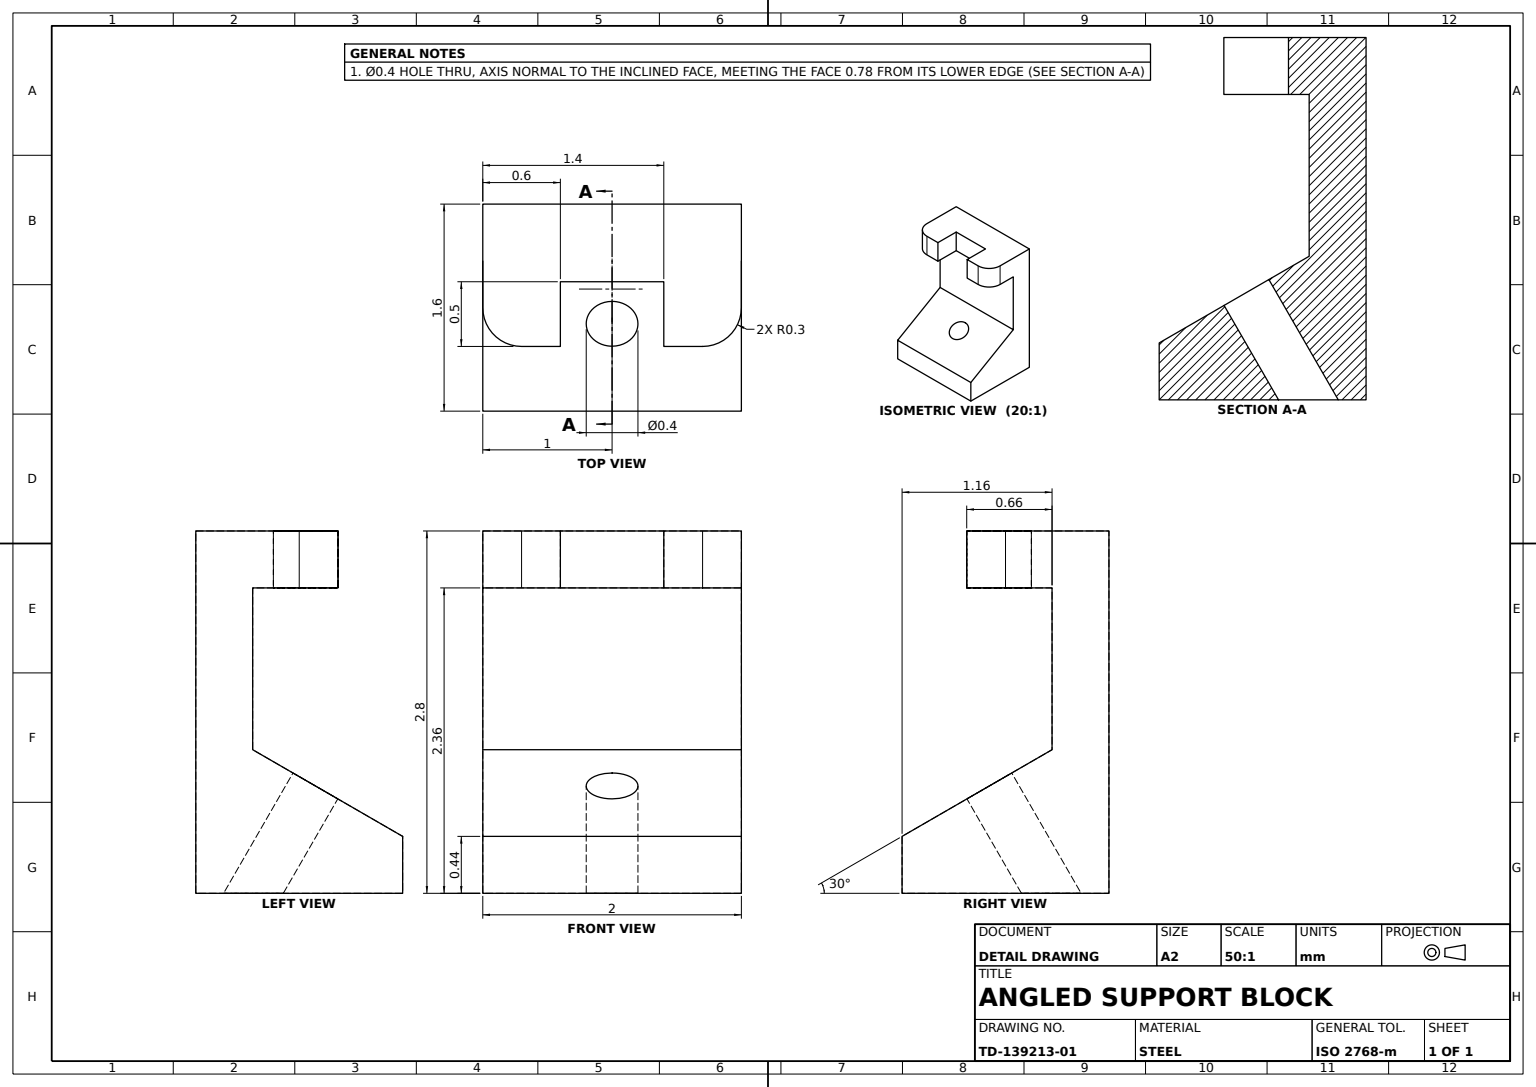
from build123d import *

# Parameters (mm, degrees)
L_BRACKET_BODY_2MM_DEPTH        = 1
UPRIGHT_SLOT_SKETCH_W           = 0.8
UPRIGHT_SLOT_SKETCH_H           = 0.5
UPRIGHT_SLOT_CUT_1MM_DEEP_DEPTH = 1
CORNER_FILLET_R0_3_A_R          = 0.3
CORNER_FILLET_R0_3_B_R          = 0.3
ANGLED_FACE_HOLE_SKETCH_R       = 0.2
ANGLED_FACE_HOLE_CUT_DEPTH      = 2


with BuildPart() as part:
    # L Profile Sketch → L Bracket Body 2mm (new, symmetric)
    with BuildSketch(Plane(origin=(0, 0, 0), x_dir=(0, 0, -1), z_dir=(1, 0, 0))):
        Polygon((0, 0), (1.6, 0), (1.6, 2.8), (0.5, 2.8), (0.5, 2.36), (1.16, 2.36), (1.16, 1.109726312), (0, 0.44), align=None)
    extrude(amount=L_BRACKET_BODY_2MM_DEPTH, both=True)

    # Upright Slot Sketch → Upright Slot Cut 1mm Deep (cut)
    with BuildSketch(Plane(origin=(0, 2.8, 0), x_dir=(1, 0, 0), z_dir=(0, 1, 0))):
        with Locations((0, 0.75)):
            Rectangle(UPRIGHT_SLOT_SKETCH_W, UPRIGHT_SLOT_SKETCH_H)
    extrude(amount=-UPRIGHT_SLOT_CUT_1MM_DEEP_DEPTH, mode=Mode.SUBTRACT)

    # Corner Fillet R0.3 A
    corner_fillet_r0_3_a_edges = [part.edges().sort_by_distance(p)[0] for p in [
        (1, 2.58, -0.5),
    ]]
    fillet(corner_fillet_r0_3_a_edges, radius=CORNER_FILLET_R0_3_A_R)

    # Corner Fillet R0.3 B
    corner_fillet_r0_3_b_edges = [part.edges().sort_by_distance(p)[0] for p in [
        (-1, 2.58, -0.5),
    ]]
    fillet(corner_fillet_r0_3_b_edges, radius=CORNER_FILLET_R0_3_B_R)

    # Angled Face Hole Sketch → Angled Face Hole Cut (cut)
    with BuildSketch(Plane(origin=(0, 0.33, 0.190525589), x_dir=(1, 0, 0), z_dir=(0, 0.8660254037844379, 0.5000000000000014))):
        with Locations(Location((0, 0.999452625, 0), (0, 0, 270))):
            Circle(ANGLED_FACE_HOLE_SKETCH_R)
    extrude(amount=-ANGLED_FACE_HOLE_CUT_DEPTH, mode=Mode.SUBTRACT)


solid = part.part
